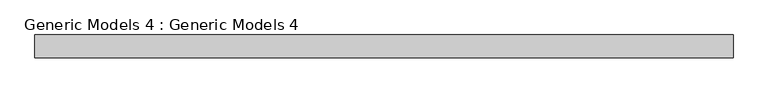
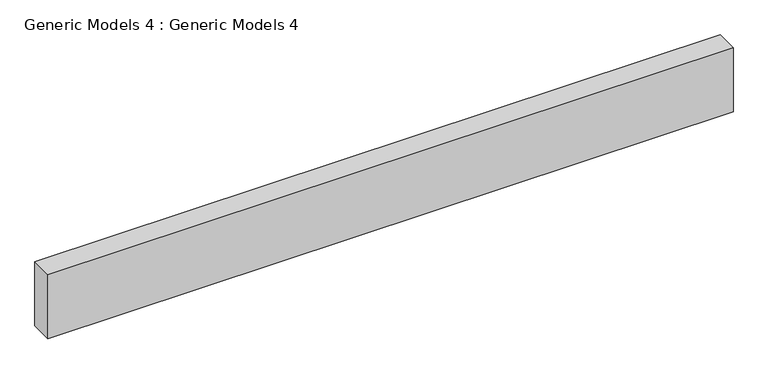
"""IFC4 building model written with IfcOpenShell, lengths in millimetres: proxy geometry, Generic Models 4 : Generic Models 4."""

from ifc_helpers import new_model, si_unit, frame, origin, place, context, project, spatial, polyline, outline, extrude, source, transform, mapped, element, save


def generic_models_4_generic_models_4_029e57d7(model_context):
    return source(origin(), model_context, "Body", "SweptSolid", [
        extrude(outline(polyline([(-5569.5456086, -11268.8679047), (-10192.3456086, -11268.8679047), (-10192.3456086, -11116.4679047), (-5569.5456086, -11116.4679047), (-5569.5456086, -11268.8679047)])), frame((0.0, 0.0, 12039.6), z_axis=(0.0, 0.0, 1.0), x_axis=(1.0, 0.0, 0.0)), (0.0, 0.0, 1.0), 457.2),
    ])


if __name__ == "__main__":
    model = new_model("IFC4")
    model_context = context("Model", 3, world=origin())
    ifc_project = project(units=[si_unit("LENGTHUNIT", "METRE", prefix="MILLI")], contexts=[model_context])
    site = spatial("IfcSite", under=ifc_project)
    building = spatial("IfcBuilding", under=site)
    placement = place(None, origin())
    generic_models_4_generic_models_4_shape = generic_models_4_generic_models_4_029e57d7(model_context)
    element("IfcBuildingElementProxy", 1, Name="Generic Models 4 : Generic Models 4", ObjectType="Generic Models 4 : Generic Models 4", at=placement, inside=building, context=model_context, shape_type="MappedRepresentation", body=[
        mapped(generic_models_4_generic_models_4_shape, transform((0.0, 0.0, 0.0), x_axis=(1.0, 0.0, 0.0), y_axis=(0.0, 1.0, 0.0), z_axis=(0.0, 0.0, 1.0))),
    ])
    save(model, "model.ifc")

# Revit data of these elements
# Element 1 (IfcBuildingElementProxy, "Generic Models 4 : Generic Models 4")
#   Materials on its faces: "WALL ACCENT 6\""
# Materials
#   "WALL ACCENT 6\"": class "Generic", colour RGB 120 120 120, transparency 0, Cost = 0
